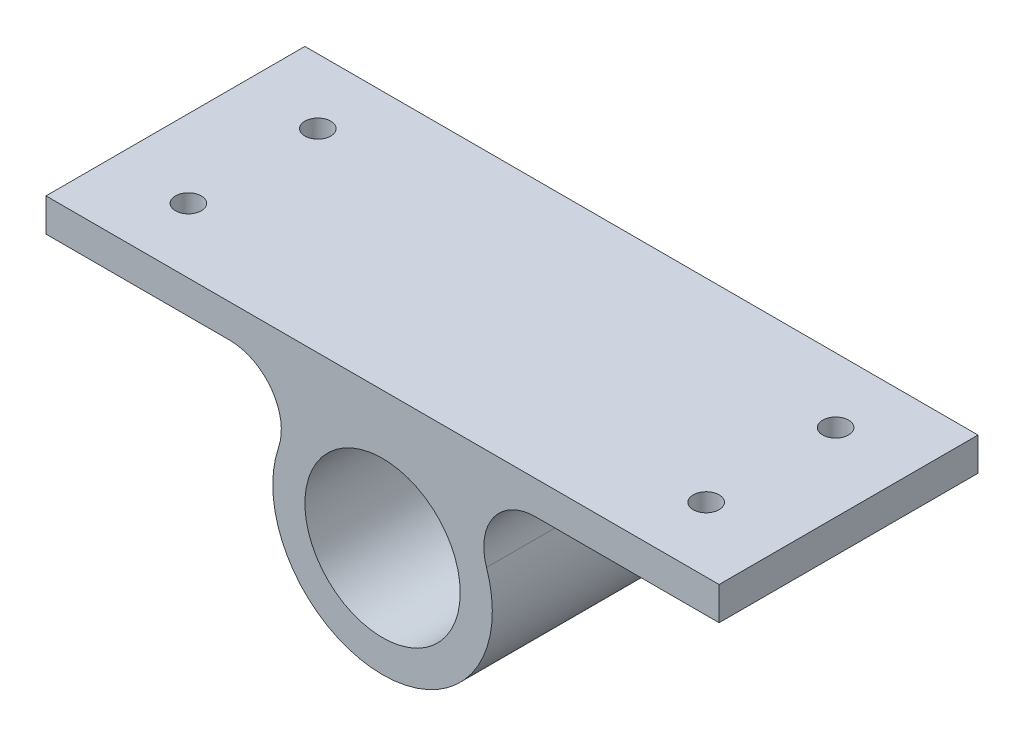
from build123d import *

# Parameters (mm, degrees)
PIVOT_BRACKET_PROFILE_R  = 75
PIVOT_BRACKET_BODY_DEPTH = 125
MOUNTING_HOLES_SKETCH_R  = 12.5
MOUNTING_HOLES_4X_DEPTH  = 125


with BuildPart() as part:
    # Pivot Bracket Profile → Pivot Bracket Body (new, symmetric)
    with BuildSketch(Plane.XY):
        with BuildLine():
            Line((147.770091697, 100), (325, 100))
            Line((325, 100), (325, 132))
            Line((325, 132), (-325, 132))
            Line((-325, 132), (-325, 100))
            Line((-325, 100), (-147.770091697, 100))
            ThreePointArc((-147.770091697, 100), (-107.142009959, 79.143763902), (-100.407882819, 33.974358974))
            ThreePointArc((-100.407882819, 33.974358974), (0, -106), (100.407882819, 33.974358974))
            ThreePointArc((100.407882819, 33.974358974), (107.142009959, 79.143763902), (147.770091697, 100))
        make_face()
        Circle(PIVOT_BRACKET_PROFILE_R, mode=Mode.SUBTRACT)
    extrude(amount=PIVOT_BRACKET_BODY_DEPTH, both=True)

    # Mounting Holes Sketch → Mounting Holes 4x (cut, symmetric)
    with BuildSketch(Plane(origin=(0, 132, 0), x_dir=(1, 0, 0), z_dir=(0, 1, 0))):
        with Locations(Location((-250, 62.5, 0), (0, 0, 270))):
            Circle(MOUNTING_HOLES_SKETCH_R)
        with Locations(Location((-250, -62.5, 0), (0, 0, 270))):
            Circle(MOUNTING_HOLES_SKETCH_R)
        with Locations(Location((250, -62.5, 0), (0, 0, 270))):
            Circle(MOUNTING_HOLES_SKETCH_R)
        with Locations(Location((250, 62.5, 0), (0, 0, 270))):
            Circle(MOUNTING_HOLES_SKETCH_R)
    extrude(amount=MOUNTING_HOLES_4X_DEPTH, both=True, mode=Mode.SUBTRACT)


solid = part.part
